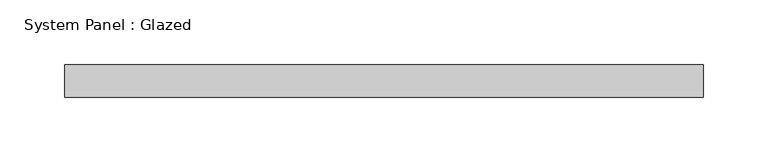
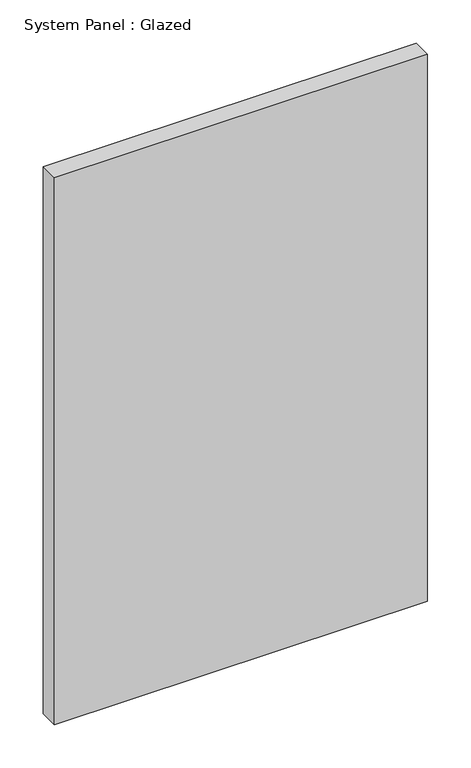
"""IFC4 building model written with IfcOpenShell, lengths in millimetres: plate geometry, System Panel : Glazed."""

from ifc_helpers import new_model, si_unit, origin, origin_with_axes, place, context, project, spatial, polyline, outline, extrude, source, transform, mapped, element, save


def system_panel_glazed_9dd6121d(model_context):
    return source(origin(), model_context, "Body", "SweptSolid", [
        extrude(outline(polyline([(247.65, 19.05), (-247.65, 19.05), (-247.65, 44.45), (247.65, 44.45), (247.65, 19.05)])), origin_with_axes(), (0.0, 0.0, 1.0), 768.35),
    ])


if __name__ == "__main__":
    model = new_model("IFC4")
    model_context = context("Model", 3, world=origin())
    ifc_project = project(units=[si_unit("LENGTHUNIT", "METRE", prefix="MILLI")], contexts=[model_context])
    site = spatial("IfcSite", under=ifc_project)
    building = spatial("IfcBuilding", under=site)
    placement = place(None, origin())
    system_panel_glazed_shape = system_panel_glazed_9dd6121d(model_context)
    element("IfcPlate", 1, ObjectType="System Panel : Glazed", at=placement, inside=building, context=model_context, shape_type="MappedRepresentation", body=[
        mapped(system_panel_glazed_shape, transform((0.0, 0.0, 0.0), x_axis=(1.0, 0.0, 0.0), y_axis=(0.0, 1.0, 0.0), z_axis=(0.0, 0.0, 1.0))),
    ])
    save(model, "model.ifc")

# Revit data of these elements
# Type "System Panel : Glazed"
#   Construction Type Id = "GSP4R"
#   Analytic Construction = "1/8 in Pilkington single glazing"
#   Visual Light Transmittance = 0.9
#   Solar Heat Gain Coefficient = 0.86
#   Heat Transfer Coefficient (U) = 1.18115 BTU/(h·ft²·°F)
#   Define Thermal Properties by = 1
# Element 1 (IfcPlate, "System Panel : Glazed")
#   Materials on its faces: "Glass"
# Materials
#   "Glass": class "Glass", colour RGB 0 128 192, transparency 0.75, Description = "Soda Lime Glass", Cost = 0
